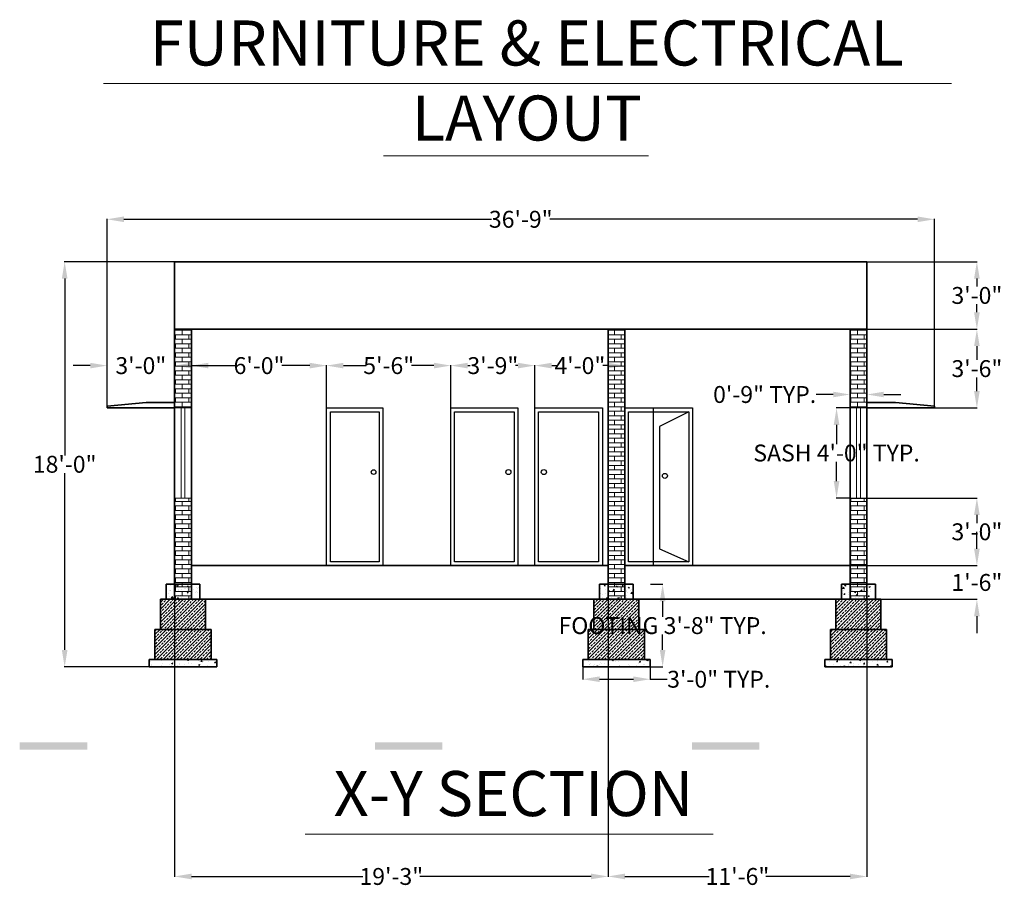
# Model space of a CAD drawing. Units: inches. Extents: x 68 to 1275, y 90 to 1276.
# Tile 3 of 6: x 627 to 1151, y 90 to 553. Entities that reach past the tile are written whole.
import ezdxf

# ---------------------------------------------------------------- set-up
doc = ezdxf.new("R2010")
doc.units = ezdxf.units.IN
doc.header["$MEASUREMENT"] = 0
for name, color, linetype, lineweight in [('A-ANNO-TEXT', 7, 'Continuous', 18), ('A-SECT', 7, 'Continuous', 35), ('A-WALL-PATT', 8, 'Continuous', 13), ('DIM', 2, 'Continuous', 18), ('DOOR', 15, 'Continuous', 25), ('S-FNDN', 7, 'Continuous', 35), ('S-FNDN-PATT', 8, 'Continuous', 13), ('WINDOW', 17, 'Continuous', 18)]:
    doc.layers.add(name, color=color, linetype=linetype, lineweight=lineweight)
doc.styles.get("Standard").update_dxf_attribs({"font": 'arial.ttf'})
doc.dimstyles.get("Standard").update_dxf_attribs({"dimtxt": 9, "dimasz": 9, "dimexe": 0.18, "dimexo": 0.0625, "dimgap": 0.09, "dimtad": 0, "dimtih": 1, "dimtoh": 1, "dimdec": 1, "dimzin": 0, "dimdsep": 46, "dimlunit": 3, "dimtxsty": 'Standard', "dimcen": 0.09, "dimadec": 0, "dimazin": 0, "dimtfac": 1, "dimtdec": 1, "dimtofl": 0, "dimtmove": 0, "dimatfit": 3, "dimfxl": 1, "dimtolj": 1, "dimtzin": 0, "dimarcsym": 0})

# ---------------------------------------------------------------- blocks, each defined once
blk = doc.blocks.new('F')
at = {"layer": 'WINDOW', "transparency": 33554531}
h = blk.add_hatch(dxfattribs=at)
h.set_pattern_fill('AR-CONC', color=256, scale=0.9)
h.paths.add_polyline_path([(109.62, -206.02), (109.62, -198.02), (91.62, -198.02), (91.62, -206.02)])
h = blk.add_hatch(dxfattribs=at)
h.set_pattern_fill('ANSI33', color=256, scale=10)
h.paths.add_polyline_path([(112.62, -222.02), (112.62, -206.02), (88.62, -206.02), (88.62, -222.02)])
h.paths.add_polyline_path([(85.62, -222.02), (85.62, -238.02), (115.62, -238.02), (115.62, -222.02)])
h = blk.add_hatch(dxfattribs=at)
h.set_pattern_fill('AR-CONC', color=256)
h.paths.add_polyline_path([(118.62, -242.02), (118.62, -238.02), (82.62, -238.02), (82.62, -242.02)])
for p, q in [((109.62, -198.02), (91.62, -198.02)), ((91.62, -198.02), (91.62, -206.02)), ((109.62, -206.02), (109.62, -198.02)), ((88.62, -206.02), (88.62, -222.02)), ((88.62, -206.02), (112.62, -206.02)), ((112.62, -222.02), (112.62, -206.02)), ((85.62, -222.02), (85.62, -238.02)), ((85.62, -222.02), (115.62, -222.02)), ((115.62, -238.02), (115.62, -222.02)), ((118.62, -238.02), (82.62, -238.02)), ((82.62, -238.02), (82.62, -242.02)), ((85.62, -238.02), (115.62, -238.02)), ((118.62, -242.02), (118.62, -238.02)), ((82.62, -242.02), (118.62, -242.02))]:
    blk.add_line(p, q)
blk = doc.blocks.new('SASH-SECTION-48IN')
for p, q in [((0, 48), (0, 0)), ((9, 48), (0, 48)), ((3.5, 48), (3.5, 0)), ((5.5, 48), (5.5, 0)), ((9, 0), (9, 48)), ((0, 0), (9, 0))]:
    blk.add_line(p, q)
blk = doc.blocks.new('*D77')
at = {"layer": 'Defpoints', "color": 0, "transparency": 16777216}
for p in [(962.75, 251.77), (969.35, 251.77), (962.75, 207.77)]:
    blk.add_point(p, dxfattribs=at)
at = {"layer": 'DIM', "color": 0, "lineweight": -2, "transparency": 16777216}
for p, q in [((962.81, 251.77), (969.53, 251.77)), ((969.35, 242.77), (969.35, 234.52)), ((969.35, 216.77), (969.35, 225.02)), ((962.81, 207.77), (969.53, 207.77))]:
    blk.add_line(p, q, dxfattribs=at)
at = {"layer": 'DIM', "color": 0, "transparency": 16777216}
for points in [[(967.85, 242.77), (970.85, 242.77), (969.35, 251.77)], [(967.85, 216.77), (970.85, 216.77), (969.35, 207.77)]]:
    blk.add_solid(points, dxfattribs=at)
at = {"layer": 'DIM', "color": 0, "transparency": 16777216, "insert": (969.35, 229.77), "char_height": 9, "attachment_point": 5}
blk.add_mtext('\\A1;FOOTING 3\'-8" TYP.', dxfattribs=at)
blk = doc.blocks.new('*D78')
at = {"layer": 'Defpoints', "color": 0, "transparency": 16777216}
for p in [(926.75, 207.77), (962.75, 207.77), (962.75, 201.17)]:
    blk.add_point(p, dxfattribs=at)
at = {"layer": 'DIM', "color": 0, "lineweight": -2, "transparency": 16777216}
for p, q in [((926.75, 207.71), (926.75, 200.99)), ((962.75, 207.71), (962.75, 200.99)), ((935.75, 201.17), (953.75, 201.17)), ((962.75, 201.17), (971.75, 201.17))]:
    blk.add_line(p, q, dxfattribs=at)
at = {"layer": 'DIM', "color": 0, "transparency": 16777216}
for points in [[(935.75, 202.67), (935.75, 199.67), (926.75, 201.17)], [(953.75, 202.67), (953.75, 199.67), (962.75, 201.17)]]:
    blk.add_solid(points, dxfattribs=at)
at = {"layer": 'DIM', "color": 0, "transparency": 16777216, "insert": (999.26, 201.17), "char_height": 9, "attachment_point": 5}
blk.add_mtext('\\A1;3\'-0" TYP.', dxfattribs=at)
blk = doc.blocks.new('*D79')
at = {"layer": 'Defpoints', "color": 0, "transparency": 16777216}
for p in [(1069.25, 345.77), (1062.05, 297.77), (1069.25, 297.77)]:
    blk.add_point(p, dxfattribs=at)
at = {"layer": 'DIM', "color": 0, "lineweight": -2, "transparency": 16777216}
for p, q in [((1069.18, 345.77), (1061.87, 345.77)), ((1062.05, 336.77), (1062.05, 326.51)), ((1062.05, 306.77), (1062.05, 317.03)), ((1069.18, 297.77), (1061.87, 297.77))]:
    blk.add_line(p, q, dxfattribs=at)
at = {"layer": 'DIM', "color": 0, "transparency": 16777216}
for points in [[(1060.55, 336.77), (1063.55, 336.77), (1062.05, 345.77)], [(1060.55, 306.77), (1063.55, 306.77), (1062.05, 297.77)]]:
    blk.add_solid(points, dxfattribs=at)
at = {"layer": 'DIM', "color": 0, "transparency": 16777216, "insert": (1062.05, 321.77), "char_height": 9, "attachment_point": 5}
blk.add_mtext('\\A1;SASH 4\'-0" TYP.', dxfattribs=at)
blk = doc.blocks.new('*D80')
at = {"layer": 'Defpoints', "color": 0, "transparency": 16777216}
for p in [(1069.25, 352.97), (1069.25, 345.77), (1078.25, 345.77)]:
    blk.add_point(p, dxfattribs=at)
at = {"layer": 'DIM', "color": 0, "lineweight": -2, "transparency": 16777216}
for p, q in [((1060.25, 352.97), (1051.25, 352.97)), ((1069.25, 345.83), (1069.25, 353.15)), ((1078.25, 345.83), (1078.25, 353.15)), ((1087.25, 352.97), (1096.25, 352.97))]:
    blk.add_line(p, q, dxfattribs=at)
at = {"layer": 'DIM', "color": 0, "transparency": 16777216}
for points in [[(1060.25, 354.47), (1060.25, 351.47), (1069.25, 352.97)], [(1087.25, 354.47), (1087.25, 351.47), (1078.25, 352.97)]]:
    blk.add_solid(points, dxfattribs=at)
at = {"layer": 'DIM', "color": 0, "transparency": 16777216, "insert": (1023.73, 352.97), "char_height": 9, "attachment_point": 5}
blk.add_mtext('\\A1;0\'-9" TYP.', dxfattribs=at)
blk = doc.blocks.new('*D99')
at = {"layer": 'Defpoints', "color": 0, "transparency": 16777216}
for p in [(1114.25, 446.37), (673.25, 345.77), (1114.25, 345.77)]:
    blk.add_point(p, dxfattribs=at)
at = {"layer": 'DIM', "color": 0, "lineweight": -2, "transparency": 16777216}
for p, q in [((673.25, 345.83), (673.25, 446.55)), ((682.25, 446.37), (878.2, 446.37)), ((1105.25, 446.37), (909.29, 446.37)), ((1114.25, 345.83), (1114.25, 446.55))]:
    blk.add_line(p, q, dxfattribs=at)
at = {"layer": 'DIM', "color": 0, "transparency": 16777216}
for points in [[(682.25, 447.87), (682.25, 444.87), (673.25, 446.37)], [(1105.25, 447.87), (1105.25, 444.87), (1114.25, 446.37)]]:
    blk.add_solid(points, dxfattribs=at)
at = {"layer": 'DIM', "color": 0, "transparency": 16777216, "insert": (893.75, 446.37), "char_height": 9, "attachment_point": 5}
blk.add_mtext('\\A1;36\'-9"', dxfattribs=at)
blk = doc.blocks.new('*D100')
at = {"layer": 'Defpoints', "color": 0, "transparency": 16777216}
for p in [(650.65, 423.77), (709.25, 423.77), (695.75, 207.77)]:
    blk.add_point(p, dxfattribs=at)
at = {"layer": 'DIM', "color": 0, "lineweight": -2, "transparency": 16777216}
for p, q in [((709.18, 423.77), (650.47, 423.77)), ((650.65, 414.77), (650.65, 320.46)), ((650.65, 216.77), (650.65, 311.09)), ((695.68, 207.77), (650.47, 207.77))]:
    blk.add_line(p, q, dxfattribs=at)
at = {"layer": 'DIM', "color": 0, "transparency": 16777216}
for points in [[(649.15, 414.77), (652.15, 414.77), (650.65, 423.77)], [(649.15, 216.77), (652.15, 216.77), (650.65, 207.77)]]:
    blk.add_solid(points, dxfattribs=at)
at = {"layer": 'DIM', "color": 0, "transparency": 16777216, "insert": (650.65, 315.77), "char_height": 9, "attachment_point": 5}
blk.add_mtext('\\A1;18\'-0"', dxfattribs=at)
blk = doc.blocks.new('*D101')
at = {"layer": 'Defpoints', "color": 0, "transparency": 16777216}
for p in [(709.246757, 368.370671), (673.246757, 345.770671), (709.246757, 345.770671)]:
    blk.add_point(p, dxfattribs=at)
at = {"layer": 'DIM', "color": 0, "lineweight": -2, "transparency": 16777216}
for p, q in [((664.246757, 368.370671), (655.246757, 368.370671)), ((673.246757, 345.833171), (673.246757, 368.550671)), ((709.246757, 345.833171), (709.246757, 368.550671)), ((718.246757, 368.370671), (727.246757, 368.370671))]:
    blk.add_line(p, q, dxfattribs=at)
at = {"layer": 'DIM', "color": 0, "transparency": 16777216}
for points in [[(664.246757, 369.870671), (664.246757, 366.870671), (673.246757, 368.370671)], [(718.246757, 369.870671), (718.246757, 366.870671), (709.246757, 368.370671)]]:
    blk.add_solid(points, dxfattribs=at)
at = {"layer": 'DIM', "color": 0, "transparency": 16777216, "insert": (691.246757, 368.370671), "char_height": 9, "attachment_point": 5}
blk.add_mtext('\\A1;3\'-0"', dxfattribs=at)
blk = doc.blocks.new('*D102')
at = {"layer": 'Defpoints', "color": 0, "transparency": 16777216}
for p in [(1078.25, 387.77), (1136.85, 387.77), (1078.25, 345.77)]:
    blk.add_point(p, dxfattribs=at)
at = {"layer": 'DIM', "color": 0, "lineweight": -2, "transparency": 16777216}
for p, q in [((1078.31, 387.77), (1137.03, 387.77)), ((1136.85, 378.77), (1136.85, 371.46)), ((1136.85, 354.77), (1136.85, 362.08)), ((1078.31, 345.77), (1137.03, 345.77))]:
    blk.add_line(p, q, dxfattribs=at)
at = {"layer": 'DIM', "color": 0, "transparency": 16777216}
for points in [[(1135.35, 378.77), (1138.35, 378.77), (1136.85, 387.77)], [(1135.35, 354.77), (1138.35, 354.77), (1136.85, 345.77)]]:
    blk.add_solid(points, dxfattribs=at)
at = {"layer": 'DIM', "color": 0, "transparency": 16777216, "insert": (1136.85, 366.77), "char_height": 9, "attachment_point": 5}
blk.add_mtext('\\A1;3\'-6"', dxfattribs=at)
blk = doc.blocks.new('*D103')
at = {"layer": 'Defpoints', "color": 0, "transparency": 16777216}
for p in [(1069.246757, 261.770671), (1136.846757, 261.770671), (1078.246757, 243.770671)]:
    blk.add_point(p, dxfattribs=at)
at = {"layer": 'DIM', "color": 0, "lineweight": -2, "transparency": 16777216}
for p, q in [((1136.846757, 270.770671), (1136.846757, 279.770671)), ((1069.309257, 261.770671), (1137.026757, 261.770671)), ((1078.309257, 243.770671), (1137.026757, 243.770671)), ((1136.846757, 234.770671), (1136.846757, 225.770671))]:
    blk.add_line(p, q, dxfattribs=at)
at = {"layer": 'DIM', "color": 0, "transparency": 16777216}
for points in [[(1135.346757, 270.770671), (1138.346757, 270.770671), (1136.846757, 261.770671)], [(1135.346757, 234.770671), (1138.346757, 234.770671), (1136.846757, 243.770671)]]:
    blk.add_solid(points, dxfattribs=at)
at = {"layer": 'DIM', "color": 0, "transparency": 16777216, "insert": (1136.846757, 252.770671), "char_height": 9, "attachment_point": 5}
blk.add_mtext('\\A1;1\'-6"', dxfattribs=at)
blk = doc.blocks.new('*D104')
at = {"layer": 'Defpoints', "color": 0, "transparency": 16777216}
for p in [(1078.25, 423.77), (1136.85, 423.77), (1078.25, 387.77)]:
    blk.add_point(p, dxfattribs=at)
at = {"layer": 'DIM', "color": 0, "lineweight": -2, "transparency": 16777216}
for p, q in [((1078.31, 423.77), (1137.03, 423.77)), ((1136.85, 414.77), (1136.85, 410.46)), ((1136.85, 396.77), (1136.85, 401.08)), ((1078.31, 387.77), (1137.03, 387.77))]:
    blk.add_line(p, q, dxfattribs=at)
at = {"layer": 'DIM', "color": 0, "transparency": 16777216}
for points in [[(1135.35, 414.77), (1138.35, 414.77), (1136.85, 423.77)], [(1135.35, 396.77), (1138.35, 396.77), (1136.85, 387.77)]]:
    blk.add_solid(points, dxfattribs=at)
at = {"layer": 'DIM', "color": 0, "transparency": 16777216, "insert": (1136.85, 405.77), "char_height": 9, "attachment_point": 5}
blk.add_mtext('\\A1;3\'-0"', dxfattribs=at)
blk = doc.blocks.new('*D105')
at = {"layer": 'Defpoints', "color": 0, "transparency": 16777216}
for p in [(1069.25, 297.77), (1136.85, 297.77), (1069.25, 261.77)]:
    blk.add_point(p, dxfattribs=at)
at = {"layer": 'DIM', "color": 0, "lineweight": -2, "transparency": 16777216}
for p, q in [((1069.31, 297.77), (1137.03, 297.77)), ((1136.85, 288.77), (1136.85, 284.46)), ((1136.85, 270.77), (1136.85, 275.08)), ((1069.31, 261.77), (1137.03, 261.77))]:
    blk.add_line(p, q, dxfattribs=at)
at = {"layer": 'DIM', "color": 0, "transparency": 16777216}
for points in [[(1135.35, 288.77), (1138.35, 288.77), (1136.85, 297.77)], [(1135.35, 270.77), (1138.35, 270.77), (1136.85, 261.77)]]:
    blk.add_solid(points, dxfattribs=at)
at = {"layer": 'DIM', "color": 0, "transparency": 16777216, "insert": (1136.85, 279.77), "char_height": 9, "attachment_point": 5}
blk.add_mtext('\\A1;3\'-0"', dxfattribs=at)
blk = doc.blocks.new('*D106')
at = {"layer": 'Defpoints', "color": 0, "transparency": 16777216}
for p in [(709.25, 387.77), (940.25, 387.77), (940.25, 96.03)]:
    blk.add_point(p, dxfattribs=at)
at = {"layer": 'DIM', "color": 0, "lineweight": -2, "transparency": 16777216}
for p, q in [((709.25, 387.71), (709.25, 95.85)), ((940.25, 387.71), (940.25, 95.85)), ((718.25, 96.03), (809.62, 96.03)), ((931.25, 96.03), (839.87, 96.03))]:
    blk.add_line(p, q, dxfattribs=at)
at = {"layer": 'DIM', "color": 0, "transparency": 16777216}
for points in [[(718.25, 97.53), (718.25, 94.53), (709.25, 96.03)], [(931.25, 97.53), (931.25, 94.53), (940.25, 96.03)]]:
    blk.add_solid(points, dxfattribs=at)
at = {"layer": 'DIM', "color": 0, "transparency": 16777216, "insert": (824.75, 96.03), "char_height": 9, "attachment_point": 5}
blk.add_mtext('\\A1;19\'-3"', dxfattribs=at)
blk = doc.blocks.new('*D107')
at = {"layer": 'Defpoints', "color": 0, "transparency": 16777216}
for p in [(940.25, 387.77), (1078.25, 387.77), (1078.25, 96.03)]:
    blk.add_point(p, dxfattribs=at)
at = {"layer": 'DIM', "color": 0, "lineweight": -2, "transparency": 16777216}
for p, q in [((940.25, 387.71), (940.25, 95.85)), ((1078.25, 387.71), (1078.25, 95.85)), ((949.25, 96.03), (994.12, 96.03)), ((1069.25, 96.03), (1024.37, 96.03))]:
    blk.add_line(p, q, dxfattribs=at)
at = {"layer": 'DIM', "color": 0, "transparency": 16777216}
for points in [[(949.25, 97.53), (949.25, 94.53), (940.25, 96.03)], [(1069.25, 97.53), (1069.25, 94.53), (1078.25, 96.03)]]:
    blk.add_solid(points, dxfattribs=at)
at = {"layer": 'DIM', "color": 0, "transparency": 16777216, "insert": (1009.25, 96.03), "char_height": 9, "attachment_point": 5}
blk.add_mtext('\\A1;11\'-6"', dxfattribs=at)
blk = doc.blocks.new('*D108')
at = {"layer": 'Defpoints', "color": 0, "transparency": 16777216}
for p in [(790.25, 368.37), (718.25, 345.77), (790.25, 345.77)]:
    blk.add_point(p, dxfattribs=at)
at = {"layer": 'DIM', "color": 0, "lineweight": -2, "transparency": 16777216}
for p, q in [((718.25, 345.83), (718.25, 368.55)), ((727.25, 368.37), (742.17, 368.37)), ((781.25, 368.37), (766.32, 368.37)), ((790.25, 345.83), (790.25, 368.55))]:
    blk.add_line(p, q, dxfattribs=at)
at = {"layer": 'DIM', "color": 0, "transparency": 16777216}
for points in [[(727.25, 369.87), (727.25, 366.87), (718.25, 368.37)], [(781.25, 369.87), (781.25, 366.87), (790.25, 368.37)]]:
    blk.add_solid(points, dxfattribs=at)
at = {"layer": 'DIM', "color": 0, "transparency": 16777216, "insert": (754.25, 368.37), "char_height": 9, "attachment_point": 5}
blk.add_mtext('\\A1;6\'-0"', dxfattribs=at)
blk = doc.blocks.new('*D109')
at = {"layer": 'Defpoints', "color": 0, "transparency": 16777216}
for p in [(856.49, 368.37), (790.25, 345.77), (856.49, 345.77)]:
    blk.add_point(p, dxfattribs=at)
at = {"layer": 'DIM', "color": 0, "lineweight": -2, "transparency": 16777216}
for p, q in [((790.25, 345.83), (790.25, 368.55)), ((799.25, 368.37), (811.31, 368.37)), ((847.49, 368.37), (835.42, 368.37)), ((856.49, 345.83), (856.49, 368.55))]:
    blk.add_line(p, q, dxfattribs=at)
at = {"layer": 'DIM', "color": 0, "transparency": 16777216}
for points in [[(799.25, 369.87), (799.25, 366.87), (790.25, 368.37)], [(847.49, 369.87), (847.49, 366.87), (856.49, 368.37)]]:
    blk.add_solid(points, dxfattribs=at)
at = {"layer": 'DIM', "color": 0, "transparency": 16777216, "insert": (823.37, 368.37), "char_height": 9, "attachment_point": 5}
blk.add_mtext('\\A1;5\'-6"', dxfattribs=at)
blk = doc.blocks.new('*D110')
at = {"layer": 'Defpoints', "color": 0, "transparency": 16777216}
for p in [(901.25, 368.37), (856.49, 345.77), (901.25, 345.77)]:
    blk.add_point(p, dxfattribs=at)
at = {"layer": 'DIM', "color": 0, "lineweight": -2, "transparency": 16777216}
for p, q in [((856.49, 345.83), (856.49, 368.55)), ((865.49, 368.37), (866.82, 368.37)), ((892.25, 368.37), (890.92, 368.37)), ((901.25, 345.83), (901.25, 368.55))]:
    blk.add_line(p, q, dxfattribs=at)
at = {"layer": 'DIM', "color": 0, "transparency": 16777216}
for points in [[(865.49, 369.87), (865.49, 366.87), (856.49, 368.37)], [(892.25, 369.87), (892.25, 366.87), (901.25, 368.37)]]:
    blk.add_solid(points, dxfattribs=at)
at = {"layer": 'DIM', "color": 0, "transparency": 16777216, "insert": (878.87, 368.37), "char_height": 9, "attachment_point": 5}
blk.add_mtext('\\A1;3\'-9"', dxfattribs=at)
blk = doc.blocks.new('*D111')
at = {"layer": 'Defpoints', "color": 0, "transparency": 16777216}
for p in [(949.25, 368.37), (901.25, 345.77), (949.25, 345.77)]:
    blk.add_point(p, dxfattribs=at)
at = {"layer": 'DIM', "color": 0, "lineweight": -2, "transparency": 16777216}
for p, q in [((901.25, 345.83), (901.25, 368.55)), ((910.25, 368.37), (913.01, 368.37)), ((940.25, 368.37), (937.48, 368.37)), ((949.25, 345.83), (949.25, 368.55))]:
    blk.add_line(p, q, dxfattribs=at)
at = {"layer": 'DIM', "color": 0, "transparency": 16777216}
for points in [[(910.25, 369.87), (910.25, 366.87), (901.25, 368.37)], [(940.25, 369.87), (940.25, 366.87), (949.25, 368.37)]]:
    blk.add_solid(points, dxfattribs=at)
at = {"layer": 'DIM', "color": 0, "transparency": 16777216, "insert": (925.25, 368.37), "char_height": 9, "attachment_point": 5}
blk.add_mtext('\\A1;4\'-0"', dxfattribs=at)

msp = doc.modelspace()

# ---------------------------------------------------------------- hatches: boundary and pattern name
at = {"layer": 'A-WALL-PATT', "transparency": 33554531}
h = msp.add_hatch(dxfattribs=at)
h.set_pattern_fill('AR-BRSTD', color=256, scale=0.9)
h.set_pattern_definition([(0, (544.0547, 449.6163), (0, 2.4003), []), (90, (544.0547, 449.6163), (-3.6, 2.4003), [2.4003, -2.4003])])
h.paths.add_polyline_path([(709.25, 345.77), (718.25, 345.77), (718.25, 387.77), (709.25, 387.77)])
h.paths.add_polyline_path([(718.25, 297.77), (709.25, 297.77), (709.25, 243.77), (718.25, 243.77)])
h.paths.add_polyline_path([(940.25, 243.77), (949.25, 243.77), (949.25, 387.77), (940.25, 387.77)])
h.paths.add_polyline_path([(1069.25, 345.77), (1078.25, 345.77), (1078.25, 387.77), (1069.25, 387.77)])
h.paths.add_polyline_path([(1069.25, 243.77), (1078.25, 243.77), (1078.25, 297.77), (1069.25, 297.77)])
at = {"layer": 'S-FNDN-PATT', "transparency": 33554567}
h = msp.add_hatch(dxfattribs=at)
h.set_pattern_fill('AR-CONC', color=256, scale=0.6)
h.set_pattern_definition([(50, (-932.027, -193.2293), (4.303561, -0.376513), [0.45, -4.95]), (355, (-932.027, -193.2293), (-0.832508, 4.513153), [0.36, -3.96]), (100.45144, (-931.6683, -193.2607), (3.471053, 4.13664), [0.382441, -4.206853]), (46.1842, (-932.027, -192.0293), (6.403448, -0.993116), [0.675, -7.425]), (96.63564, (-931.4933, -192.112), (5.607972, 5.844712), [0.573662, -6.310283]), (351.18416, (-932.027, -192.029), (5.607972, 5.844712), [0.54, -5.94]), (21, (-931.427, -192.3293), (3.581442, -2.4157133), [0.45, -4.95]), (326, (-931.427, -192.3293), (1.459892, 4.3509), [0.36, -3.96]), (71.45144, (-931.1285, -192.5306), (5.041334, 1.935187), [0.382441, -4.206853]), (37.5, (-932.027, -193.2293), (0.0729591, 1.9973631), [0, -3.912, 0, -4.02, 0, -3.975]), (7.5, (-932.027, -193.2293), (1.5784172, 2.3664703), [0, -2.292, 0, -3.822, 0, -1.515]), (327.5, (-933.365, -193.2293), (3.2029346, -0.1353292), [0, -1.5, 0, -4.68, 0, -6.21]), (317.5, (-933.965, -193.2293), (3.499117, 0.60063), [0, -1.95, 0, -3.108, 0, -4.41])])
h.paths.add_polyline_path([(662.68, 163.59), (662.68, 167.59), (626.68, 167.59), (626.68, 163.59)])
h.paths.add_polyline_path([(851.98, 163.59), (851.98, 167.59), (815.98, 167.59), (815.98, 163.59)])
h.paths.add_polyline_path([(1020.98, 163.59), (1020.98, 167.59), (984.98, 167.59), (984.98, 163.59)])

# ---------------------------------------------------------------- linework, layer by layer
at = {"layer": 'A-ANNO-TEXT'}
for p, q in [((671.42, 518.76), (1123.32, 518.76)), ((820.51, 480.18), (961.74, 480.18)), ((778.75, 118.63), (996.32, 118.63))]:
    msp.add_line(p, q, dxfattribs=at)
at = {"layer": 'A-SECT'}
for p, q in [((709.25, 243.77), (709.25, 423.77)), ((709.25, 423.77), (1078.25, 423.77)), ((1078.25, 243.77), (1078.25, 423.77)), ((709.25, 387.77), (1078.25, 387.77)), ((718.25, 243.77), (718.25, 387.77)), ((940.25, 243.77), (940.25, 387.77)), ((949.25, 243.77), (949.25, 387.77)), ((1069.25, 243.77), (1069.25, 387.77)), ((694.07, 348.77), (673.25, 346.77)), ((673.25, 345.77), (673.25, 346.77)), ((709.25, 348.77), (694.07, 348.77)), ((709.25, 345.77), (709.25, 348.77)), ((1078.25, 348.77), (1093.42, 348.77)), ((1093.42, 348.77), (1114.25, 346.77)), ((1114.25, 345.77), (1114.25, 346.77)), ((709.25, 345.77), (673.25, 345.77)), ((1078.25, 345.77), (1114.25, 345.77)), ((718.25, 261.77), (940.25, 261.77)), ((949.25, 261.77), (1069.25, 261.77)), ((709.25, 243.77), (1078.25, 243.77)), ((709.25, 243.77), (718.25, 243.77)), ((940.25, 243.77), (949.25, 243.77)), ((1069.25, 243.77), (1078.25, 243.77))]:
    msp.add_line(p, q, dxfattribs=at)
at = {"layer": 'DOOR'}
for p, q in [((964.25, 345.77), (964.25, 261.77)), ((983.31, 343.77), (967.74, 335.96)), ((967.74, 335.96), (967.74, 270.65)), ((967.74, 270.65), (983.31, 263.77))]:
    msp.add_line(p, q, dxfattribs=at)
for points in [[(790.25, 345.77), (820.25, 345.77), (820.25, 261.77), (790.25, 261.77)], [(792.25, 343.77), (818.25, 343.77), (818.25, 263.77), (792.25, 263.77)], [(856.49, 345.77), (892.25, 345.77), (892.25, 261.77), (856.49, 261.77)], [(858.49, 343.77), (890.25, 343.77), (890.25, 263.77), (858.49, 263.77)], [(901.25, 345.77), (937.26, 345.77), (937.26, 261.77), (901.25, 261.77)], [(903.25, 343.77), (935.26, 343.77), (935.26, 263.77), (903.25, 263.77)], [(949.25, 345.77), (985.31, 345.77), (985.31, 261.77), (949.25, 261.77)], [(951.25, 343.77), (983.31, 343.77), (983.31, 263.77), (951.25, 263.77)]]:
    msp.add_lwpolyline(points, close=True, dxfattribs=at)
for centre, radius in [((815.29, 311.62), 1.23), ((887.15, 311.62), 1.38), ((906.04, 311.62), 1.38), ((970.59, 309.58), 1.32)]:
    msp.add_circle(centre, radius, dxfattribs=at)

# ---------------------------------------------------------------- block references
at = {"layer": 'S-FNDN'}
for p in [(613.12, 449.79), (844.12, 449.79), (973.12, 449.79)]:
    msp.add_blockref('F', p, dxfattribs=at)
at = {"layer": 'WINDOW'}
msp.add_blockref('SASH-SECTION-48IN', (709.25, 297.77), dxfattribs=at)
at = {"layer": 'WINDOW', "rotation": 180}
msp.add_blockref('SASH-SECTION-48IN', (1078.25, 345.77), dxfattribs=at)

# ---------------------------------------------------------------- texts
at = {"layer": 'A-ANNO-TEXT', "char_height": 24, "attachment_point": 2}
for s, width, insert in [('FURNITURE & ELECTRICAL LAYOUT', 501.3778, (896.93, 552.35)), ('X-Y SECTION', 255.8943, (889.83, 152.22))]:
    msp.add_mtext_dynamic_manual_height_columns(s, width=width, gutter_width=1, heights=[0], dxfattribs=dict(at, insert=insert))

# ---------------------------------------------------------------- dimensions: what is measured, and where the dimension line sits
at = {"layer": 'DIM'}
for base, p1, p2, picture, middle in [((1114.25, 446.37), (673.25, 345.77), (1114.25, 345.77), '*D99', (893.75, 446.37)), ((940.25, 96.03), (709.25, 387.77), (940.25, 387.77), '*D106', (824.75, 96.03)), ((1078.25, 96.03), (940.25, 387.77), (1078.25, 387.77), '*D107', (1009.25, 96.03)), ((709.25, 368.37), (673.25, 345.77), (709.25, 345.77), '*D101', (691.25, 368.37)), ((790.25, 368.37), (718.25, 345.77), (790.25, 345.77), '*D108', (754.25, 368.37)), ((856.49, 368.37), (790.25, 345.77), (856.49, 345.77), '*D109', (823.37, 368.37)), ((901.25, 368.37), (856.49, 345.77), (901.25, 345.77), '*D110', (878.87, 368.37)), ((949.25, 368.37), (901.25, 345.77), (949.25, 345.77), '*D111', (925.25, 368.37))]:
    dim = msp.add_linear_dim(base=base, p1=p1, p2=p2, dimstyle='Standard', override={"dimdec": 1, "dimlfac": 1, "dimrnd": 0, "dimzin": 1, "dimdsep": 46, "dimlunit": 4, "dimfrac": 2}, dxfattribs=at)
    dim.commit()
    dim.dimension.update_dxf_attribs({"geometry": picture, "text_midpoint": middle})
for base, p1, p2, picture, middle in [((650.65, 423.77), (695.75, 207.77), (709.25, 423.77), '*D100', (650.65, 315.77)), ((1136.85, 423.77), (1078.25, 387.77), (1078.25, 423.77), '*D104', (1136.85, 405.77)), ((1136.85, 387.77), (1078.25, 345.77), (1078.25, 387.77), '*D102', (1136.85, 366.77)), ((1136.85, 297.77), (1069.25, 261.77), (1069.25, 297.77), '*D105', (1136.85, 279.77)), ((1136.85, 261.77), (1078.25, 243.77), (1069.25, 261.77), '*D103', (1136.85, 252.77))]:
    dim = msp.add_linear_dim(base=base, p1=p1, p2=p2, angle=90, dimstyle='Standard', override={"dimdec": 1, "dimlfac": 1, "dimrnd": 0, "dimzin": 1, "dimdsep": 46, "dimlunit": 4, "dimfrac": 2}, dxfattribs=at)
    dim.commit()
    dim.dimension.update_dxf_attribs({"geometry": picture, "text_midpoint": middle})
for base, p1, p2, angle, text, picture, middle in [((1069.25, 352.97), (1078.25, 345.77), (1069.25, 345.77), 180, '<> TYP.', '*D80', (1023.73, 352.97)), ((1062.05, 297.77), (1069.25, 345.77), (1069.25, 297.77), 270, 'SASH <> TYP.', '*D79', (1062.05, 321.77)), ((969.35, 251.77), (962.75, 207.77), (962.75, 251.77), 90, 'FOOTING <> TYP.', '*D77', (969.35, 229.77))]:
    dim = msp.add_linear_dim(base=base, p1=p1, p2=p2, angle=angle, text=text, dimstyle='Standard', override={"dimdec": 1, "dimlfac": 1, "dimrnd": 0, "dimzin": 1, "dimdsep": 46, "dimlunit": 4, "dimfrac": 2}, dxfattribs=at)
    dim.commit()
    dim.dimension.update_dxf_attribs({"geometry": picture, "text_midpoint": middle})
dim = msp.add_linear_dim(base=(962.75, 201.17), p1=(926.75, 207.77), p2=(962.75, 207.77), text='<> TYP.', dimstyle='Standard', override={"dimdec": 1, "dimlfac": 1, "dimrnd": 0, "dimzin": 1, "dimdsep": 46, "dimlunit": 4, "dimfrac": 2}, dxfattribs=at)
dim.commit()
dim.dimension.update_dxf_attribs({"geometry": '*D78', "text_midpoint": (999.26, 201.17)})

doc.saveas('drawing.dxf')
